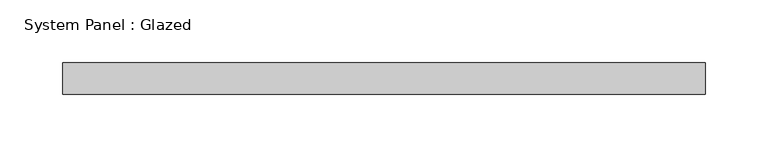
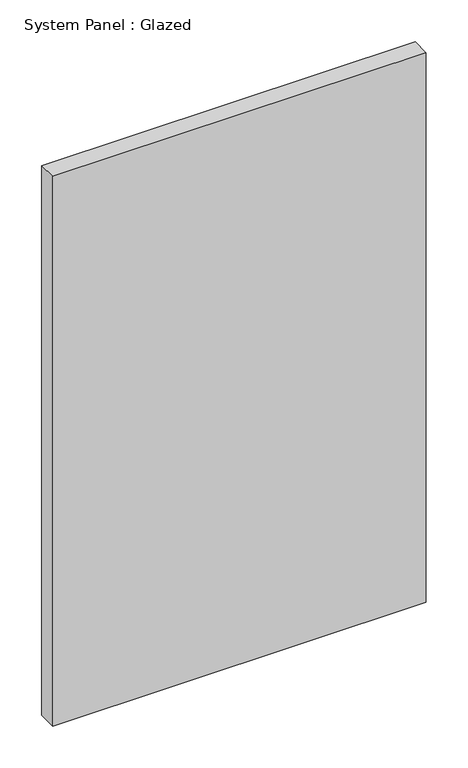
"""IFC4 building model written with IfcOpenShell, lengths in millimetres: plate geometry, System Panel : Glazed."""

from ifc_helpers import new_model, si_unit, origin, origin_with_axes, place, context, project, spatial, polyline, outline, extrude, source, transform, mapped, element, save


def system_panel_glazed_29e6fa37(model_context):
    return source(origin(), model_context, "Body", "SweptSolid", [
        extrude(outline(polyline([(257.175, 19.05), (-257.175, 19.05), (-257.175, 44.45), (257.175, 44.45), (257.175, 19.05)])), origin_with_axes(), (0.0, 0.0, 1.0), 799.6990947),
    ])


if __name__ == "__main__":
    model = new_model("IFC4")
    model_context = context("Model", 3, world=origin())
    ifc_project = project(units=[si_unit("LENGTHUNIT", "METRE", prefix="MILLI")], contexts=[model_context])
    site = spatial("IfcSite", under=ifc_project)
    building = spatial("IfcBuilding", under=site)
    placement = place(None, origin())
    system_panel_glazed_shape = system_panel_glazed_29e6fa37(model_context)
    element("IfcPlate", 1, ObjectType="System Panel : Glazed", at=placement, inside=building, context=model_context, shape_type="MappedRepresentation", body=[
        mapped(system_panel_glazed_shape, transform((0.0, 0.0, 0.0), x_axis=(1.0, 0.0, 0.0), y_axis=(0.0, 1.0, 0.0), z_axis=(0.0, 0.0, 1.0))),
    ])
    save(model, "model.ifc")

# Revit data of these elements
# Type "System Panel : Glazed"
#   Construction Type Id = "GSP4R"
#   Analytic Construction = "1/8 in Pilkington single glazing"
#   Visual Light Transmittance = 0.9
#   Solar Heat Gain Coefficient = 0.86
#   Heat Transfer Coefficient (U) = 1.18115 BTU/(h·ft²·°F)
#   Define Thermal Properties by = 1
# Element 1 (IfcPlate, "System Panel : Glazed")
#   Materials on its faces: "Glass"
# Materials
#   "Glass": class "Glass", colour RGB 0 128 192, transparency 0.75, Description = "Soda Lime Glass", Cost = 0
